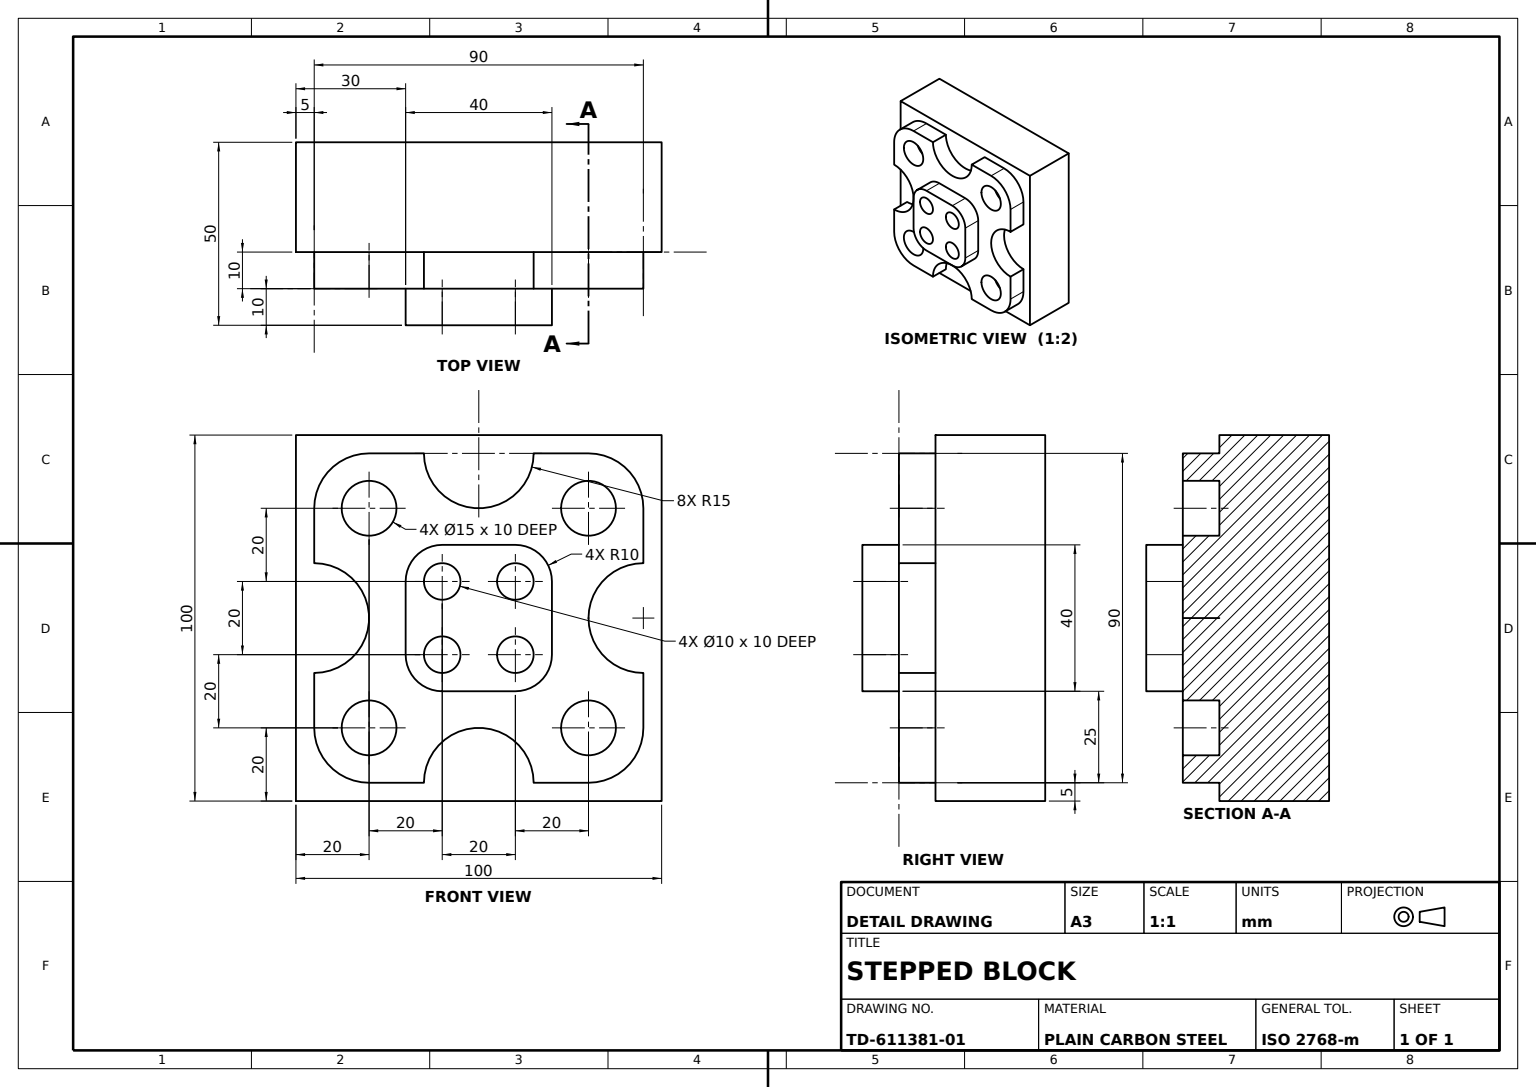
from build123d import *

# Parameters (mm, degrees)
BASE_BLOCK_100X100X30_DEPTH        = 15
LOCATING_PADS_10MM_DEPTH           = 10
LOCATING_PAD_FILLET_R15_1_R        = 15
LOCATING_PAD_FILLET_R15_2_R        = 15
LOCATING_PAD_FILLET_R15_3_R        = 15
LOCATING_PAD_FILLET_R15_4_R        = 15
RAISED_PAD_10MM_DEPTH              = 10
RAISED_PAD_FILLET_R10_1_R          = 10
RAISED_PAD_FILLET_R10_2_R          = 10
RAISED_PAD_FILLET_R10_3_R          = 10
RAISED_PAD_FILLET_R10_4_R          = 10
RAISED_PAD_POCKET_SKETCH_R         = 5
RAISED_PAD_POCKET_10X10X10_DEPTH   = 10
LOCATING_PAD_POCKET_SKETCH_R       = 7.5
LOCATING_PAD_POCKET_15X15X10_DEPTH = 10


with BuildPart() as part:
    # Base Block Sketch → Base Block 100x100x30 (new, symmetric)
    with BuildSketch(Plane.XY):
        Polygon((50, 45), (-50, 45), (-50, -55), (50, -55), (50, 0), align=None)
    extrude(amount=BASE_BLOCK_100X100X30_DEPTH, both=True)

    # Locating Pads Sketch → Locating Pads 10mm (add)
    with BuildSketch(Plane(origin=(0, 0, -15), x_dir=(-1, 0, 0), z_dir=(0, 0, -1))):
        with BuildLine():
            Line((15, 40), (45, 40))
            Line((45, 40), (45, 10))
            ThreePointArc((45, 10), (30, -5), (45, -20))
            Line((45, -20), (45, -50))
            Line((45, -50), (15, -50))
            ThreePointArc((15, -50), (0, -35), (-15, -50))
            Line((-15, -50), (-45, -50))
            Line((-45, -50), (-45, -20))
            ThreePointArc((-45, -20), (-30, -5), (-45, 10))
            Line((-45, 10), (-45, 40))
            Line((-45, 40), (-15, 40))
            ThreePointArc((-15, 40), (0, 25), (15, 40))
        make_face()
    extrude(amount=LOCATING_PADS_10MM_DEPTH)

    # Locating Pad Fillet R15 1
    locating_pad_fillet_r15_1_edges = [part.edges().sort_by_distance(p)[0] for p in [
        (-45, -50, -20),
    ]]
    fillet(locating_pad_fillet_r15_1_edges, radius=LOCATING_PAD_FILLET_R15_1_R)

    # Locating Pad Fillet R15 2
    locating_pad_fillet_r15_2_edges = [part.edges().sort_by_distance(p)[0] for p in [
        (45, -50, -20),
    ]]
    fillet(locating_pad_fillet_r15_2_edges, radius=LOCATING_PAD_FILLET_R15_2_R)

    # Locating Pad Fillet R15 3
    locating_pad_fillet_r15_3_edges = [part.edges().sort_by_distance(p)[0] for p in [
        (45, 40, -20),
    ]]
    fillet(locating_pad_fillet_r15_3_edges, radius=LOCATING_PAD_FILLET_R15_3_R)

    # Locating Pad Fillet R15 4
    locating_pad_fillet_r15_4_edges = [part.edges().sort_by_distance(p)[0] for p in [
        (-45, 40, -20),
    ]]
    fillet(locating_pad_fillet_r15_4_edges, radius=LOCATING_PAD_FILLET_R15_4_R)

    # Raised Pad Sketch → Raised Pad 10mm (add)
    with BuildSketch(Plane(origin=(0, 0, -25), x_dir=(-1, 0, 0), z_dir=(0, 0, -1))):
        Polygon((0, -25), (20, -25), (20, 15), (-20, 15), (-20, -25), align=None)
    extrude(amount=RAISED_PAD_10MM_DEPTH)

    # Raised Pad Fillet R10 1
    raised_pad_fillet_r10_1_edges = [part.edges().sort_by_distance(p)[0] for p in [
        (20, -25, -30),
    ]]
    fillet(raised_pad_fillet_r10_1_edges, radius=RAISED_PAD_FILLET_R10_1_R)

    # Raised Pad Fillet R10 2
    raised_pad_fillet_r10_2_edges = [part.edges().sort_by_distance(p)[0] for p in [
        (20, 15, -30),
    ]]
    fillet(raised_pad_fillet_r10_2_edges, radius=RAISED_PAD_FILLET_R10_2_R)

    # Raised Pad Fillet R10 3
    raised_pad_fillet_r10_3_edges = [part.edges().sort_by_distance(p)[0] for p in [
        (-20, 15, -30),
    ]]
    fillet(raised_pad_fillet_r10_3_edges, radius=RAISED_PAD_FILLET_R10_3_R)

    # Raised Pad Fillet R10 4
    raised_pad_fillet_r10_4_edges = [part.edges().sort_by_distance(p)[0] for p in [
        (-20, -25, -30),
    ]]
    fillet(raised_pad_fillet_r10_4_edges, radius=RAISED_PAD_FILLET_R10_4_R)

    # Raised Pad Pocket Sketch → Raised Pad Pocket 10x10x10 (cut)
    with BuildSketch(Plane(origin=(0, 0, -35), x_dir=(-1, 0, 0), z_dir=(0, 0, -1))):
        with Locations((10, 5)):
            Circle(RAISED_PAD_POCKET_SKETCH_R)
        with Locations((10, -15)):
            Circle(RAISED_PAD_POCKET_SKETCH_R)
        with Locations((-10, -15)):
            Circle(RAISED_PAD_POCKET_SKETCH_R)
        with Locations((-10, 5)):
            Circle(RAISED_PAD_POCKET_SKETCH_R)
    extrude(amount=-RAISED_PAD_POCKET_10X10X10_DEPTH, mode=Mode.SUBTRACT)

    # Locating Pad Pocket Sketch → Locating Pad Pocket 15x15x10 (cut)
    with BuildSketch(Plane(origin=(0, 0, -25), x_dir=(-1, 0, 0), z_dir=(0, 0, -1))):
        with Locations((30, 25)):
            Circle(LOCATING_PAD_POCKET_SKETCH_R)
        with Locations((30, -35)):
            Circle(LOCATING_PAD_POCKET_SKETCH_R)
        with Locations((-30, -35)):
            Circle(LOCATING_PAD_POCKET_SKETCH_R)
        with Locations((-30, 25)):
            Circle(LOCATING_PAD_POCKET_SKETCH_R)
    extrude(amount=-LOCATING_PAD_POCKET_15X15X10_DEPTH, mode=Mode.SUBTRACT)


solid = part.part
